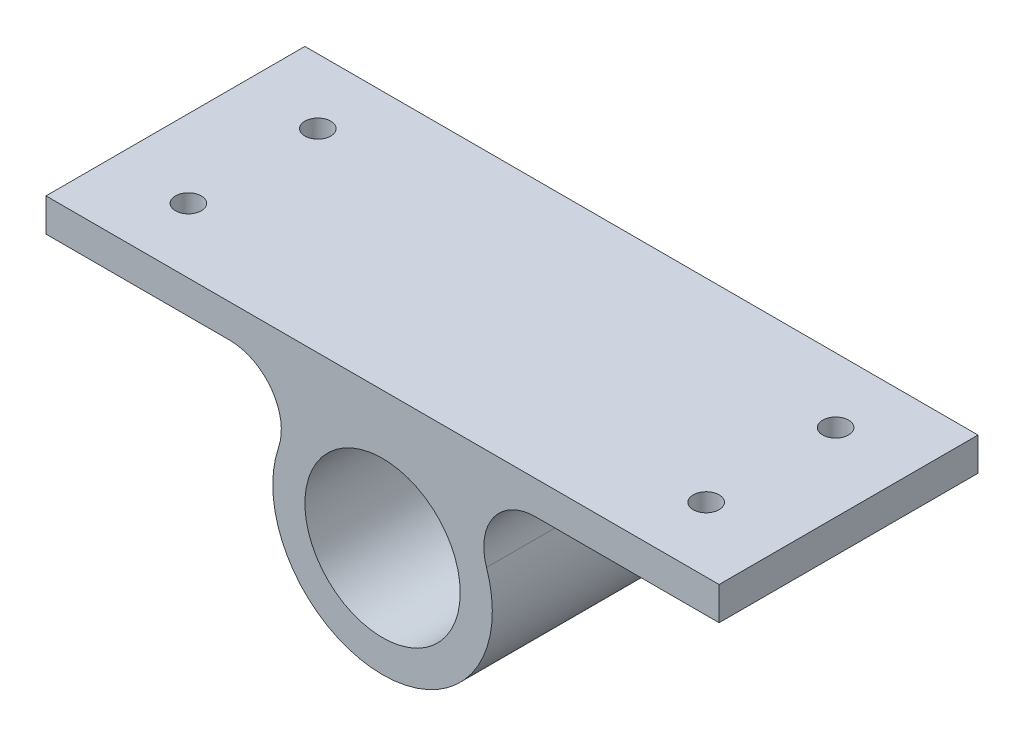
ISO-10303-21;
HEADER;
FILE_DESCRIPTION(('STEP AP214'),'2;1');
FILE_NAME('part.step','',(''),(''),'','','');
FILE_SCHEMA(('AUTOMOTIVE_DESIGN { 1 0 10303 214 1 1 1 1 }'));
ENDSEC;
DATA;
#1=APPLICATION_CONTEXT('core data for automotive mechanical design processes');
#2=APPLICATION_PROTOCOL_DEFINITION('international standard','automotive_design',2000,#1);
#3=PRODUCT_CONTEXT('',#1,'mechanical');
#4=PRODUCT('Part','Part','',(#3));
#5=PRODUCT_RELATED_PRODUCT_CATEGORY('part','',(#4));
#6=PRODUCT_DEFINITION_FORMATION('','',#4);
#7=PRODUCT_DEFINITION_CONTEXT('part definition',#1,'design');
#8=PRODUCT_DEFINITION('design','',#6,#7);
#9=PRODUCT_DEFINITION_SHAPE('','',#8);
#10=(LENGTH_UNIT() NAMED_UNIT(*) SI_UNIT(.MILLI.,.METRE.));
#11=(NAMED_UNIT(*) PLANE_ANGLE_UNIT() SI_UNIT($,.RADIAN.));
#12=(NAMED_UNIT(*) SI_UNIT($,.STERADIAN.) SOLID_ANGLE_UNIT());
#13=UNCERTAINTY_MEASURE_WITH_UNIT(LENGTH_MEASURE(1.E-05),#10,'distance_accuracy_value','');
#14=(GEOMETRIC_REPRESENTATION_CONTEXT(3) GLOBAL_UNCERTAINTY_ASSIGNED_CONTEXT((#13)) GLOBAL_UNIT_ASSIGNED_CONTEXT((#10,
#11,#12)) REPRESENTATION_CONTEXT('',''));
#15=CARTESIAN_POINT('',(0.,0.,0.));
#16=DIRECTION('',(0.,0.,1.));
#17=DIRECTION('',(1.,0.,0.));
#18=AXIS2_PLACEMENT_3D('',#15,#16,#17);
#19=CARTESIAN_POINT('',(147.770091696527,50.,125.));
#20=DIRECTION('',(0.,0.,1.));
#21=DIRECTION('',(1.,0.,0.));
#22=AXIS2_PLACEMENT_3D('',#19,#20,#21);
#23=PLANE('',#22);
#24=DIRECTION('',(0.,1.,0.));
#25=VECTOR('',#24,1.);
#26=CARTESIAN_POINT('',(325.,132.,125.));
#27=LINE('',#26,#25);
#28=CARTESIAN_POINT('',(325.,100.,125.));
#29=VERTEX_POINT('',#28);
#30=CARTESIAN_POINT('',(325.,132.,125.));
#31=VERTEX_POINT('',#30);
#32=EDGE_CURVE('E153',#29,#31,#27,.T.);
#33=ORIENTED_EDGE('',*,*,#32,.T.);
#34=DIRECTION('',(-1.,0.,0.));
#35=VECTOR('',#34,1.);
#36=CARTESIAN_POINT('',(-325.,132.,125.));
#37=LINE('',#36,#35);
#38=CARTESIAN_POINT('',(-325.,132.,125.));
#39=VERTEX_POINT('',#38);
#40=EDGE_CURVE('E101',#31,#39,#37,.T.);
#41=ORIENTED_EDGE('',*,*,#40,.T.);
#42=DIRECTION('',(0.,-1.,0.));
#43=VECTOR('',#42,1.);
#44=CARTESIAN_POINT('',(-325.,132.,125.));
#45=LINE('',#44,#43);
#46=CARTESIAN_POINT('',(-325.,100.,125.));
#47=VERTEX_POINT('',#46);
#48=EDGE_CURVE('E194',#39,#47,#45,.T.);
#49=ORIENTED_EDGE('',*,*,#48,.T.);
#50=DIRECTION('',(1.,0.,0.));
#51=VECTOR('',#50,1.);
#52=CARTESIAN_POINT('',(-325.,100.,125.));
#53=LINE('',#52,#51);
#54=CARTESIAN_POINT('',(-147.770091696527,100.,125.));
#55=VERTEX_POINT('',#54);
#56=EDGE_CURVE('E197',#47,#55,#53,.T.);
#57=ORIENTED_EDGE('',*,*,#56,.T.);
#58=CARTESIAN_POINT('',(-147.770091696527,50.,125.));
#59=DIRECTION('',(0.,0.,-1.));
#60=DIRECTION('',(1.,0.,0.));
#61=AXIS2_PLACEMENT_3D('',#58,#59,#60);
#62=CIRCLE('',#61,50.);
#63=CARTESIAN_POINT('',(-100.407882819435,33.974358974359,125.));
#64=VERTEX_POINT('',#63);
#65=EDGE_CURVE('E119',#55,#64,#62,.T.);
#66=ORIENTED_EDGE('',*,*,#65,.T.);
#67=CARTESIAN_POINT('',(0.,0.,125.));
#68=DIRECTION('',(0.,0.,1.));
#69=DIRECTION('',(1.,0.,0.));
#70=AXIS2_PLACEMENT_3D('',#67,#68,#69);
#71=CIRCLE('',#70,106.);
#72=CARTESIAN_POINT('',(100.407882819435,33.974358974359,125.));
#73=VERTEX_POINT('',#72);
#74=EDGE_CURVE('E111',#64,#73,#71,.T.);
#75=ORIENTED_EDGE('',*,*,#74,.T.);
#76=CARTESIAN_POINT('',(147.770091696527,50.,125.));
#77=DIRECTION('',(0.,0.,-1.));
#78=DIRECTION('',(1.,0.,0.));
#79=AXIS2_PLACEMENT_3D('',#76,#77,#78);
#80=CIRCLE('',#79,50.);
#81=CARTESIAN_POINT('',(147.770091696527,100.,125.));
#82=VERTEX_POINT('',#81);
#83=EDGE_CURVE('E117',#73,#82,#80,.T.);
#84=ORIENTED_EDGE('',*,*,#83,.T.);
#85=DIRECTION('',(1.,0.,0.));
#86=VECTOR('',#85,1.);
#87=CARTESIAN_POINT('',(147.770091696527,100.,125.));
#88=LINE('',#87,#86);
#89=EDGE_CURVE('E59',#82,#29,#88,.T.);
#90=ORIENTED_EDGE('',*,*,#89,.T.);
#91=EDGE_LOOP('',(#33,#41,#49,#57,#66,#75,#84,#90));
#92=FACE_BOUND('',#91,.T.);
#93=CARTESIAN_POINT('',(0.,0.,125.));
#94=DIRECTION('',(0.,0.,1.));
#95=DIRECTION('',(1.,0.,0.));
#96=AXIS2_PLACEMENT_3D('',#93,#94,#95);
#97=CIRCLE('',#96,75.);
#98=CARTESIAN_POINT('',(75.,0.,125.));
#99=VERTEX_POINT('',#98);
#100=EDGE_CURVE('E142',#99,#99,#97,.T.);
#101=ORIENTED_EDGE('',*,*,#100,.F.);
#102=EDGE_LOOP('',(#101));
#103=FACE_BOUND('',#102,.T.);
#104=ADVANCED_FACE('F39',(#92,#103),#23,.T.);
#105=CARTESIAN_POINT('',(147.770091696527,50.,-125.));
#106=DIRECTION('',(0.,0.,1.));
#107=DIRECTION('',(1.,0.,0.));
#108=AXIS2_PLACEMENT_3D('',#105,#106,#107);
#109=PLANE('',#108);
#110=DIRECTION('',(0.,1.,0.));
#111=VECTOR('',#110,1.);
#112=CARTESIAN_POINT('',(325.,132.,-125.));
#113=LINE('',#112,#111);
#114=CARTESIAN_POINT('',(325.,100.,-125.));
#115=VERTEX_POINT('',#114);
#116=CARTESIAN_POINT('',(325.,132.,-125.));
#117=VERTEX_POINT('',#116);
#118=EDGE_CURVE('E137',#115,#117,#113,.T.);
#119=ORIENTED_EDGE('',*,*,#118,.F.);
#120=DIRECTION('',(1.,0.,0.));
#121=VECTOR('',#120,1.);
#122=CARTESIAN_POINT('',(147.770091696527,100.,-125.));
#123=LINE('',#122,#121);
#124=CARTESIAN_POINT('',(147.770091696527,100.,-125.));
#125=VERTEX_POINT('',#124);
#126=EDGE_CURVE('E91',#125,#115,#123,.T.);
#127=ORIENTED_EDGE('',*,*,#126,.F.);
#128=CARTESIAN_POINT('',(147.770091696527,50.,-125.));
#129=DIRECTION('',(0.,0.,-1.));
#130=DIRECTION('',(1.,0.,0.));
#131=AXIS2_PLACEMENT_3D('',#128,#129,#130);
#132=CIRCLE('',#131,50.);
#133=CARTESIAN_POINT('',(100.407882819435,33.974358974359,-125.));
#134=VERTEX_POINT('',#133);
#135=EDGE_CURVE('E87',#134,#125,#132,.T.);
#136=ORIENTED_EDGE('',*,*,#135,.F.);
#137=CARTESIAN_POINT('',(0.,0.,-125.));
#138=DIRECTION('',(0.,0.,1.));
#139=DIRECTION('',(1.,0.,0.));
#140=AXIS2_PLACEMENT_3D('',#137,#138,#139);
#141=CIRCLE('',#140,106.);
#142=CARTESIAN_POINT('',(-100.407882819435,33.974358974359,-125.));
#143=VERTEX_POINT('',#142);
#144=EDGE_CURVE('E126',#143,#134,#141,.T.);
#145=ORIENTED_EDGE('',*,*,#144,.F.);
#146=CARTESIAN_POINT('',(-147.770091696527,50.,-125.));
#147=DIRECTION('',(0.,0.,-1.));
#148=DIRECTION('',(1.,0.,0.));
#149=AXIS2_PLACEMENT_3D('',#146,#147,#148);
#150=CIRCLE('',#149,50.);
#151=CARTESIAN_POINT('',(-147.770091696527,100.,-125.));
#152=VERTEX_POINT('',#151);
#153=EDGE_CURVE('E146',#152,#143,#150,.T.);
#154=ORIENTED_EDGE('',*,*,#153,.F.);
#155=DIRECTION('',(1.,0.,0.));
#156=VECTOR('',#155,1.);
#157=CARTESIAN_POINT('',(-325.,100.,-125.));
#158=LINE('',#157,#156);
#159=CARTESIAN_POINT('',(-325.,100.,-125.));
#160=VERTEX_POINT('',#159);
#161=EDGE_CURVE('E148',#160,#152,#158,.T.);
#162=ORIENTED_EDGE('',*,*,#161,.F.);
#163=DIRECTION('',(0.,-1.,0.));
#164=VECTOR('',#163,1.);
#165=CARTESIAN_POINT('',(-325.,132.,-125.));
#166=LINE('',#165,#164);
#167=CARTESIAN_POINT('',(-325.,132.,-125.));
#168=VERTEX_POINT('',#167);
#169=EDGE_CURVE('E145',#168,#160,#166,.T.);
#170=ORIENTED_EDGE('',*,*,#169,.F.);
#171=DIRECTION('',(-1.,0.,0.));
#172=VECTOR('',#171,1.);
#173=CARTESIAN_POINT('',(-325.,132.,-125.));
#174=LINE('',#173,#172);
#175=EDGE_CURVE('E143',#117,#168,#174,.T.);
#176=ORIENTED_EDGE('',*,*,#175,.F.);
#177=EDGE_LOOP('',(#119,#127,#136,#145,#154,#162,#170,#176));
#178=FACE_BOUND('',#177,.T.);
#179=CARTESIAN_POINT('',(0.,0.,-125.));
#180=DIRECTION('',(0.,0.,1.));
#181=DIRECTION('',(1.,0.,0.));
#182=AXIS2_PLACEMENT_3D('',#179,#180,#181);
#183=CIRCLE('',#182,75.);
#184=CARTESIAN_POINT('',(75.,0.,-125.));
#185=VERTEX_POINT('',#184);
#186=EDGE_CURVE('E187',#185,#185,#183,.T.);
#187=ORIENTED_EDGE('',*,*,#186,.T.);
#188=EDGE_LOOP('',(#187));
#189=FACE_BOUND('',#188,.T.);
#190=ADVANCED_FACE('F209',(#178,#189),#109,.F.);
#191=CARTESIAN_POINT('',(325.,132.,125.));
#192=DIRECTION('',(-1.,0.,0.));
#193=DIRECTION('',(0.,-1.,0.));
#194=AXIS2_PLACEMENT_3D('',#191,#192,#193);
#195=PLANE('',#194);
#196=ORIENTED_EDGE('',*,*,#118,.T.);
#197=DIRECTION('',(0.,0.,-1.));
#198=VECTOR('',#197,1.);
#199=CARTESIAN_POINT('',(325.,132.,125.));
#200=LINE('',#199,#198);
#201=EDGE_CURVE('E11',#31,#117,#200,.T.);
#202=ORIENTED_EDGE('',*,*,#201,.F.);
#203=ORIENTED_EDGE('',*,*,#32,.F.);
#204=DIRECTION('',(0.,0.,-1.));
#205=VECTOR('',#204,1.);
#206=CARTESIAN_POINT('',(325.,100.,125.));
#207=LINE('',#206,#205);
#208=EDGE_CURVE('E133',#29,#115,#207,.T.);
#209=ORIENTED_EDGE('',*,*,#208,.T.);
#210=EDGE_LOOP('',(#196,#202,#203,#209));
#211=FACE_BOUND('',#210,.T.);
#212=ADVANCED_FACE('F41',(#211),#195,.F.);
#213=CARTESIAN_POINT('',(-325.,132.,125.));
#214=DIRECTION('',(0.,-1.,0.));
#215=DIRECTION('',(0.,0.,-1.));
#216=AXIS2_PLACEMENT_3D('',#213,#214,#215);
#217=PLANE('',#216);
#218=CARTESIAN_POINT('',(250.,132.,-62.5));
#219=DIRECTION('',(0.,-1.,0.));
#220=DIRECTION('',(0.,0.,-1.));
#221=AXIS2_PLACEMENT_3D('',#218,#219,#220);
#222=CIRCLE('',#221,12.5);
#223=CARTESIAN_POINT('',(250.,132.,-75.));
#224=VERTEX_POINT('',#223);
#225=EDGE_CURVE('E171',#224,#224,#222,.T.);
#226=ORIENTED_EDGE('',*,*,#225,.T.);
#227=EDGE_LOOP('',(#226));
#228=FACE_BOUND('',#227,.T.);
#229=CARTESIAN_POINT('',(250.,132.,62.5));
#230=DIRECTION('',(0.,-1.,0.));
#231=DIRECTION('',(0.,0.,-1.));
#232=AXIS2_PLACEMENT_3D('',#229,#230,#231);
#233=CIRCLE('',#232,12.5);
#234=CARTESIAN_POINT('',(250.,132.,50.));
#235=VERTEX_POINT('',#234);
#236=EDGE_CURVE('E169',#235,#235,#233,.T.);
#237=ORIENTED_EDGE('',*,*,#236,.T.);
#238=EDGE_LOOP('',(#237));
#239=FACE_BOUND('',#238,.T.);
#240=CARTESIAN_POINT('',(-250.,132.,62.5));
#241=DIRECTION('',(0.,-1.,0.));
#242=DIRECTION('',(0.,0.,-1.));
#243=AXIS2_PLACEMENT_3D('',#240,#241,#242);
#244=CIRCLE('',#243,12.5);
#245=CARTESIAN_POINT('',(-250.,132.,50.));
#246=VERTEX_POINT('',#245);
#247=EDGE_CURVE('E183',#246,#246,#244,.T.);
#248=ORIENTED_EDGE('',*,*,#247,.T.);
#249=EDGE_LOOP('',(#248));
#250=FACE_BOUND('',#249,.T.);
#251=CARTESIAN_POINT('',(-250.,132.,-62.5));
#252=DIRECTION('',(0.,-1.,0.));
#253=DIRECTION('',(0.,0.,-1.));
#254=AXIS2_PLACEMENT_3D('',#251,#252,#253);
#255=CIRCLE('',#254,12.5);
#256=CARTESIAN_POINT('',(-250.,132.,-75.));
#257=VERTEX_POINT('',#256);
#258=EDGE_CURVE('E173',#257,#257,#255,.T.);
#259=ORIENTED_EDGE('',*,*,#258,.T.);
#260=EDGE_LOOP('',(#259));
#261=FACE_BOUND('',#260,.T.);
#262=ORIENTED_EDGE('',*,*,#175,.T.);
#263=DIRECTION('',(0.,0.,-1.));
#264=VECTOR('',#263,1.);
#265=CARTESIAN_POINT('',(-325.,132.,125.));
#266=LINE('',#265,#264);
#267=EDGE_CURVE('E47',#39,#168,#266,.T.);
#268=ORIENTED_EDGE('',*,*,#267,.F.);
#269=ORIENTED_EDGE('',*,*,#40,.F.);
#270=ORIENTED_EDGE('',*,*,#201,.T.);
#271=EDGE_LOOP('',(#262,#268,#269,#270));
#272=FACE_BOUND('',#271,.T.);
#273=ADVANCED_FACE('F259',(#228,#239,#250,#261,#272),#217,.F.);
#274=CARTESIAN_POINT('',(-325.,132.,125.));
#275=DIRECTION('',(1.,0.,0.));
#276=DIRECTION('',(0.,0.,-1.));
#277=AXIS2_PLACEMENT_3D('',#274,#275,#276);
#278=PLANE('',#277);
#279=ORIENTED_EDGE('',*,*,#169,.T.);
#280=DIRECTION('',(0.,0.,-1.));
#281=VECTOR('',#280,1.);
#282=CARTESIAN_POINT('',(-325.,100.,125.));
#283=LINE('',#282,#281);
#284=EDGE_CURVE('E159',#47,#160,#283,.T.);
#285=ORIENTED_EDGE('',*,*,#284,.F.);
#286=ORIENTED_EDGE('',*,*,#48,.F.);
#287=ORIENTED_EDGE('',*,*,#267,.T.);
#288=EDGE_LOOP('',(#279,#285,#286,#287));
#289=FACE_BOUND('',#288,.T.);
#290=ADVANCED_FACE('F265',(#289),#278,.F.);
#291=CARTESIAN_POINT('',(-325.,100.,125.));
#292=DIRECTION('',(0.,1.,0.));
#293=DIRECTION('',(0.,0.,1.));
#294=AXIS2_PLACEMENT_3D('',#291,#292,#293);
#295=PLANE('',#294);
#296=CARTESIAN_POINT('',(-250.,100.,62.5));
#297=DIRECTION('',(0.,1.,0.));
#298=DIRECTION('',(0.,0.,1.));
#299=AXIS2_PLACEMENT_3D('',#296,#297,#298);
#300=CIRCLE('',#299,12.5);
#301=CARTESIAN_POINT('',(-250.,100.,75.));
#302=VERTEX_POINT('',#301);
#303=EDGE_CURVE('E43',#302,#302,#300,.T.);
#304=ORIENTED_EDGE('',*,*,#303,.T.);
#305=EDGE_LOOP('',(#304));
#306=FACE_BOUND('',#305,.T.);
#307=CARTESIAN_POINT('',(-250.,100.,-62.5));
#308=DIRECTION('',(0.,1.,0.));
#309=DIRECTION('',(0.,0.,1.));
#310=AXIS2_PLACEMENT_3D('',#307,#308,#309);
#311=CIRCLE('',#310,12.5);
#312=CARTESIAN_POINT('',(-250.,100.,-50.));
#313=VERTEX_POINT('',#312);
#314=EDGE_CURVE('E175',#313,#313,#311,.T.);
#315=ORIENTED_EDGE('',*,*,#314,.T.);
#316=EDGE_LOOP('',(#315));
#317=FACE_BOUND('',#316,.T.);
#318=ORIENTED_EDGE('',*,*,#161,.T.);
#319=DIRECTION('',(0.,0.,-1.));
#320=VECTOR('',#319,1.);
#321=CARTESIAN_POINT('',(-147.770091696527,100.,125.));
#322=LINE('',#321,#320);
#323=EDGE_CURVE('E160',#55,#152,#322,.T.);
#324=ORIENTED_EDGE('',*,*,#323,.F.);
#325=ORIENTED_EDGE('',*,*,#56,.F.);
#326=ORIENTED_EDGE('',*,*,#284,.T.);
#327=EDGE_LOOP('',(#318,#324,#325,#326));
#328=FACE_BOUND('',#327,.T.);
#329=ADVANCED_FACE('F201',(#306,#317,#328),#295,.F.);
#330=CARTESIAN_POINT('',(-147.770091696527,50.,125.));
#331=DIRECTION('',(0.,0.,-1.));
#332=DIRECTION('',(-1.,0.,0.));
#333=AXIS2_PLACEMENT_3D('',#330,#331,#332);
#334=CYLINDRICAL_SURFACE('',#333,50.);
#335=ORIENTED_EDGE('',*,*,#153,.T.);
#336=DIRECTION('',(0.,0.,-1.));
#337=VECTOR('',#336,1.);
#338=CARTESIAN_POINT('',(-100.407882819435,33.974358974359,125.));
#339=LINE('',#338,#337);
#340=EDGE_CURVE('E129',#64,#143,#339,.T.);
#341=ORIENTED_EDGE('',*,*,#340,.F.);
#342=ORIENTED_EDGE('',*,*,#65,.F.);
#343=ORIENTED_EDGE('',*,*,#323,.T.);
#344=EDGE_LOOP('',(#335,#341,#342,#343));
#345=FACE_BOUND('',#344,.T.);
#346=ADVANCED_FACE('F210',(#345),#334,.F.);
#347=CARTESIAN_POINT('',(0.,0.,125.));
#348=DIRECTION('',(0.,0.,-1.));
#349=DIRECTION('',(-1.,0.,0.));
#350=AXIS2_PLACEMENT_3D('',#347,#348,#349);
#351=CYLINDRICAL_SURFACE('',#350,106.);
#352=ORIENTED_EDGE('',*,*,#144,.T.);
#353=DIRECTION('',(0.,0.,-1.));
#354=VECTOR('',#353,1.);
#355=CARTESIAN_POINT('',(100.407882819435,33.974358974359,125.));
#356=LINE('',#355,#354);
#357=EDGE_CURVE('E124',#73,#134,#356,.T.);
#358=ORIENTED_EDGE('',*,*,#357,.F.);
#359=ORIENTED_EDGE('',*,*,#74,.F.);
#360=ORIENTED_EDGE('',*,*,#340,.T.);
#361=EDGE_LOOP('',(#352,#358,#359,#360));
#362=FACE_BOUND('',#361,.T.);
#363=ADVANCED_FACE('F127',(#362),#351,.T.);
#364=CARTESIAN_POINT('',(147.770091696527,50.,125.));
#365=DIRECTION('',(0.,0.,-1.));
#366=DIRECTION('',(-1.,0.,0.));
#367=AXIS2_PLACEMENT_3D('',#364,#365,#366);
#368=CYLINDRICAL_SURFACE('',#367,50.);
#369=ORIENTED_EDGE('',*,*,#135,.T.);
#370=DIRECTION('',(0.,0.,-1.));
#371=VECTOR('',#370,1.);
#372=CARTESIAN_POINT('',(147.770091696527,100.,125.));
#373=LINE('',#372,#371);
#374=EDGE_CURVE('E128',#82,#125,#373,.T.);
#375=ORIENTED_EDGE('',*,*,#374,.F.);
#376=ORIENTED_EDGE('',*,*,#83,.F.);
#377=ORIENTED_EDGE('',*,*,#357,.T.);
#378=EDGE_LOOP('',(#369,#375,#376,#377));
#379=FACE_BOUND('',#378,.T.);
#380=ADVANCED_FACE('F135',(#379),#368,.F.);
#381=CARTESIAN_POINT('',(147.770091696527,100.,125.));
#382=DIRECTION('',(0.,1.,0.));
#383=DIRECTION('',(0.,0.,1.));
#384=AXIS2_PLACEMENT_3D('',#381,#382,#383);
#385=PLANE('',#384);
#386=CARTESIAN_POINT('',(250.,100.,-62.5));
#387=DIRECTION('',(0.,1.,0.));
#388=DIRECTION('',(0.,0.,1.));
#389=AXIS2_PLACEMENT_3D('',#386,#387,#388);
#390=CIRCLE('',#389,12.5);
#391=CARTESIAN_POINT('',(250.,100.,-50.));
#392=VERTEX_POINT('',#391);
#393=EDGE_CURVE('E166',#392,#392,#390,.T.);
#394=ORIENTED_EDGE('',*,*,#393,.T.);
#395=EDGE_LOOP('',(#394));
#396=FACE_BOUND('',#395,.T.);
#397=CARTESIAN_POINT('',(250.,100.,62.5));
#398=DIRECTION('',(0.,1.,0.));
#399=DIRECTION('',(0.,0.,1.));
#400=AXIS2_PLACEMENT_3D('',#397,#398,#399);
#401=CIRCLE('',#400,12.5);
#402=CARTESIAN_POINT('',(250.,100.,75.));
#403=VERTEX_POINT('',#402);
#404=EDGE_CURVE('E164',#403,#403,#401,.T.);
#405=ORIENTED_EDGE('',*,*,#404,.T.);
#406=EDGE_LOOP('',(#405));
#407=FACE_BOUND('',#406,.T.);
#408=ORIENTED_EDGE('',*,*,#126,.T.);
#409=ORIENTED_EDGE('',*,*,#208,.F.);
#410=ORIENTED_EDGE('',*,*,#89,.F.);
#411=ORIENTED_EDGE('',*,*,#374,.T.);
#412=EDGE_LOOP('',(#408,#409,#410,#411));
#413=FACE_BOUND('',#412,.T.);
#414=ADVANCED_FACE('F216',(#396,#407,#413),#385,.F.);
#415=CARTESIAN_POINT('',(0.,0.,125.));
#416=DIRECTION('',(0.,0.,-1.));
#417=DIRECTION('',(-1.,0.,0.));
#418=AXIS2_PLACEMENT_3D('',#415,#416,#417);
#419=CYLINDRICAL_SURFACE('',#418,75.);
#420=ORIENTED_EDGE('',*,*,#100,.T.);
#421=EDGE_LOOP('',(#420));
#422=FACE_BOUND('',#421,.T.);
#423=ORIENTED_EDGE('',*,*,#186,.F.);
#424=EDGE_LOOP('',(#423));
#425=FACE_BOUND('',#424,.T.);
#426=ADVANCED_FACE('F217',(#422,#425),#419,.F.);
#427=CARTESIAN_POINT('',(250.,7.00000000000001,62.5));
#428=DIRECTION('',(0.,1.,0.));
#429=DIRECTION('',(0.,0.,1.));
#430=AXIS2_PLACEMENT_3D('',#427,#428,#429);
#431=CYLINDRICAL_SURFACE('',#430,12.5);
#432=ORIENTED_EDGE('',*,*,#404,.F.);
#433=EDGE_LOOP('',(#432));
#434=FACE_BOUND('',#433,.T.);
#435=ORIENTED_EDGE('',*,*,#236,.F.);
#436=EDGE_LOOP('',(#435));
#437=FACE_BOUND('',#436,.T.);
#438=ADVANCED_FACE('F226',(#434,#437),#431,.F.);
#439=CARTESIAN_POINT('',(250.,7.00000000000001,-62.5));
#440=DIRECTION('',(0.,1.,0.));
#441=DIRECTION('',(0.,0.,1.));
#442=AXIS2_PLACEMENT_3D('',#439,#440,#441);
#443=CYLINDRICAL_SURFACE('',#442,12.5);
#444=ORIENTED_EDGE('',*,*,#393,.F.);
#445=EDGE_LOOP('',(#444));
#446=FACE_BOUND('',#445,.T.);
#447=ORIENTED_EDGE('',*,*,#225,.F.);
#448=EDGE_LOOP('',(#447));
#449=FACE_BOUND('',#448,.T.);
#450=ADVANCED_FACE('F242',(#446,#449),#443,.F.);
#451=CARTESIAN_POINT('',(-250.,7.00000000000001,-62.5));
#452=DIRECTION('',(0.,1.,0.));
#453=DIRECTION('',(0.,0.,1.));
#454=AXIS2_PLACEMENT_3D('',#451,#452,#453);
#455=CYLINDRICAL_SURFACE('',#454,12.5);
#456=ORIENTED_EDGE('',*,*,#314,.F.);
#457=EDGE_LOOP('',(#456));
#458=FACE_BOUND('',#457,.T.);
#459=ORIENTED_EDGE('',*,*,#258,.F.);
#460=EDGE_LOOP('',(#459));
#461=FACE_BOUND('',#460,.T.);
#462=ADVANCED_FACE('F239',(#458,#461),#455,.F.);
#463=CARTESIAN_POINT('',(-250.,7.00000000000001,62.5));
#464=DIRECTION('',(0.,1.,0.));
#465=DIRECTION('',(0.,0.,1.));
#466=AXIS2_PLACEMENT_3D('',#463,#464,#465);
#467=CYLINDRICAL_SURFACE('',#466,12.5);
#468=ORIENTED_EDGE('',*,*,#303,.F.);
#469=EDGE_LOOP('',(#468));
#470=FACE_BOUND('',#469,.T.);
#471=ORIENTED_EDGE('',*,*,#247,.F.);
#472=EDGE_LOOP('',(#471));
#473=FACE_BOUND('',#472,.T.);
#474=ADVANCED_FACE('F245',(#470,#473),#467,.F.);
#475=CLOSED_SHELL('',(#104,#190,#212,#273,#290,#329,#346,#363,#380,#414,#426,#438,#450,#462,#474));
#476=MANIFOLD_SOLID_BREP('B2',#475);
#477=ADVANCED_BREP_SHAPE_REPRESENTATION('',(#18,#476),#14);
#478=SHAPE_DEFINITION_REPRESENTATION(#9,#477);
ENDSEC;
END-ISO-10303-21;
